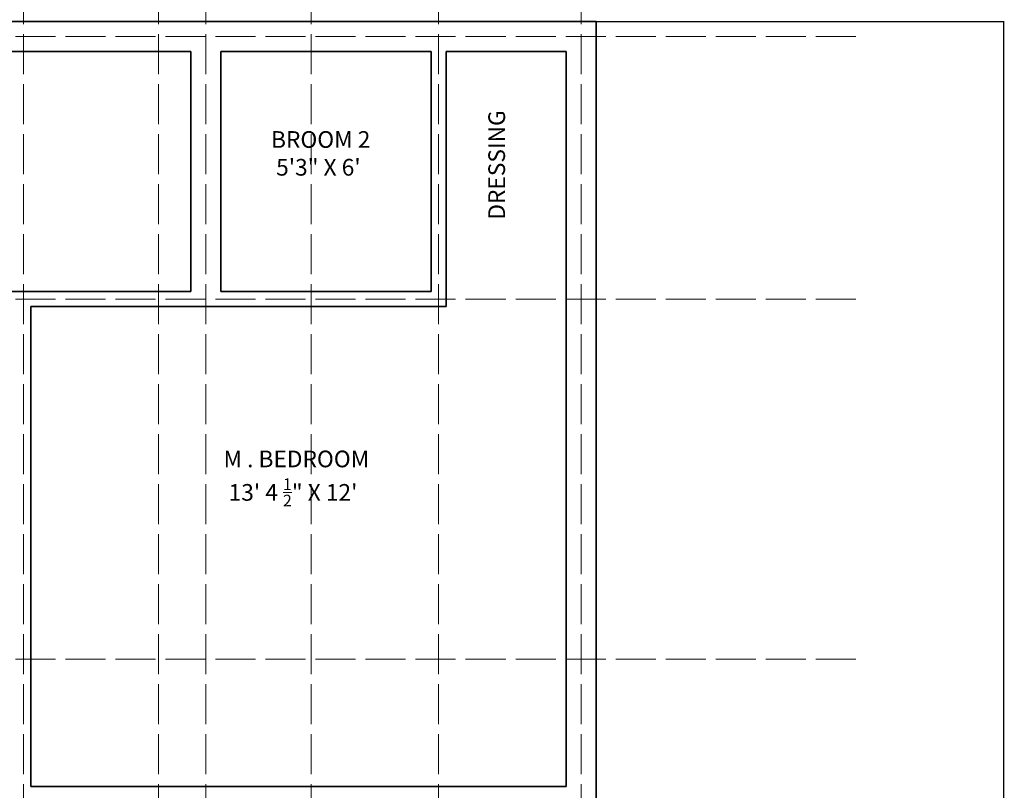
# Model space of a CAD drawing. Units: inches. Extents: x 1159 to 4240, y 1112 to 2085.
# Tile 9 of 13: x 1535 to 1831, y 1737 to 1968. Entities that reach past the tile are written whole.
import ezdxf

# ---------------------------------------------------------------- set-up
doc = ezdxf.new("R2010")
doc.units = ezdxf.units.IN
doc.linetypes.add('ACAD_ISO02W100', pattern=[15, 12, -3])
for name, color, linetype, lineweight in [('A-ANNO-DIMS', 2, 'Continuous', 18), ('A-AREA-IDEN', 30, 'Continuous', 18), ('A-GRID', 8, 'ACAD_ISO02W100', 13), ('WALL', 7, 'Continuous', 35)]:
    doc.layers.add(name, color=color, linetype=linetype, lineweight=lineweight)
doc.styles.get("Standard").update_dxf_attribs({"font": 'arial.ttf'})
doc.dimstyles.get("Standard").update_dxf_attribs({"dimtxt": 0.18, "dimasz": 0.18, "dimexe": 0.18, "dimexo": 0.0625, "dimgap": 0.09, "dimtad": 0, "dimtih": 1, "dimtoh": 1, "dimdec": 4, "dimzin": 0, "dimdsep": 46, "dimtxsty": 'Standard', "dimcen": 0.09, "dimadec": 0, "dimazin": 0, "dimtfac": 1, "dimtdec": 4, "dimtofl": 0, "dimtmove": 0, "dimatfit": 3, "dimfxl": 1, "dimtolj": 1, "dimtzin": 0, "dimarcsym": 0})

# ---------------------------------------------------------------- blocks, each defined once
blk = doc.blocks.new('HOUSE-35x60-WALL-LAYOUT')
for p, q in [((0, 720), (420, 720)), ((420, 720), (420, 297)), ((121.5, 711), (298.5, 711)), ((298.5, 711), (298.5, 639)), ((307.5, 711), (307.5, 639)), ((307.5, 711), (370.5, 711)), ((370.5, 711), (370.5, 639)), ((375, 711), (375, 634.5)), ((375, 711), (411, 711)), ((411, 711), (411, 634.5)), ((121.5, 639), (298.5, 639)), ((307.5, 639), (370.5, 639)), ((250.5, 634.5), (250.5, 490.5)), ((250.5, 634.5), (375, 634.5)), ((411, 634.5), (411, 490.5)), ((250.5, 490.5), (411, 490.5))]:
    blk.add_line(p, q)
blk = doc.blocks.new('HOUSE-35x60-SETTING-OUT-GRID')
for p, q in [((333.07, 0), (333.07, 883.25)), ((373.57, 0), (373.57, 883.25)), ((387.82, 0), (387.82, 883.25)), ((419.32, 0), (419.32, 883.25)), ((457.57, 0), (457.57, 883.25)), ((500.32, 0), (500.32, 883.25)), ((582.7, 806.25), (0, 806.25)), ((582.7, 727.5), (0, 727.5)), ((582.7, 619.5), (0, 619.5))]:
    blk.add_line(p, q)
blk = doc.blocks.new('*D23')
at = {"layer": 'A-ANNO-DIMS', "color": 0, "lineweight": -2, "transparency": 16777216}
for p, q in [((1708.19, 1967.7), (1830.54, 1967.7)), ((1830.36, 1967.52), (1830.36, 1607.88)), ((1830.36, 1247.88), (1830.36, 1607.52)), ((1708.19, 1247.7), (1830.54, 1247.7))]:
    blk.add_line(p, q, dxfattribs=at)
at = {"layer": 'A-ANNO-DIMS', "color": 0, "lineweight": 100, "transparency": 16777216}
for points in [[(1830.33, 1967.52), (1830.39, 1967.52), (1830.36, 1967.7)], [(1830.33, 1247.88), (1830.39, 1247.88), (1830.36, 1247.7)]]:
    blk.add_solid(points, dxfattribs=at)
at = {"layer": 'Defpoints', "color": 0, "lineweight": 100, "transparency": 16777216}
for p in [(1708.13, 1967.7), (1830.36, 1967.7), (1708.13, 1247.7)]:
    blk.add_point(p, dxfattribs=at)
at = {"layer": 'A-ANNO-DIMS', "color": 0, "transparency": 16777216, "insert": (1830.36, 1607.7), "char_height": 0.18, "attachment_point": 5}
blk.add_mtext('\\A1;720', dxfattribs=at)

msp = doc.modelspace()

# ---------------------------------------------------------------- block references
at = {"layer": 'A-GRID'}
msp.add_blockref('HOUSE-35x60-SETTING-OUT-GRID', (1203.31, 1156.954), dxfattribs=at)
at = {"layer": 'WALL'}
msp.add_blockref('HOUSE-35x60-WALL-LAYOUT', (1288.126, 1247.702), dxfattribs=at)

# ---------------------------------------------------------------- texts
at = {"layer": 'A-AREA-IDEN', "insert": (1675.814, 1908.276), "char_height": 5, "attachment_point": 1, "rotation": 90}
msp.add_mtext_dynamic_manual_height_columns('\\A1;DRESSING', width=140.18614, gutter_width=12.5, heights=[0], dxfattribs=at)
at = {"layer": 'A-AREA-IDEN', "char_height": 5, "attachment_point": 1}
for s, insert in [('\\A1;BROOM 2\\P 5\'3" X 6\'', (1610.638, 1934.831)), ('\\A1;M . BEDROOM\\P 13\' 4 {\\H0.7x;\\S1/2;}" X 12\'', (1596.39, 1838.992))]:
    msp.add_mtext_dynamic_manual_height_columns(s, width=140.18614, gutter_width=12.5, heights=[0], dxfattribs=dict(at, insert=insert))

# ---------------------------------------------------------------- dimensions: what is measured, and where the dimension line sits
at = {"layer": 'A-ANNO-DIMS'}
dim = msp.add_linear_dim(base=(1830.364, 1967.702), p1=(1708.125, 1247.702), p2=(1708.125, 1967.702), angle=90, dimstyle='Standard', override={"dimdec": 0, "dimlfac": 1, "dimrnd": 0, "dimzin": 0, "dimdsep": 46, "dimlunit": 2}, dxfattribs=at)
dim.commit()
dim.dimension.update_dxf_attribs({"geometry": '*D23', "text_midpoint": (1830.364, 1607.702)})

doc.saveas('drawing.dxf')
